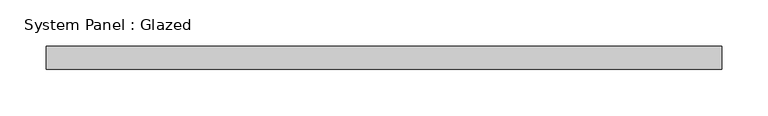
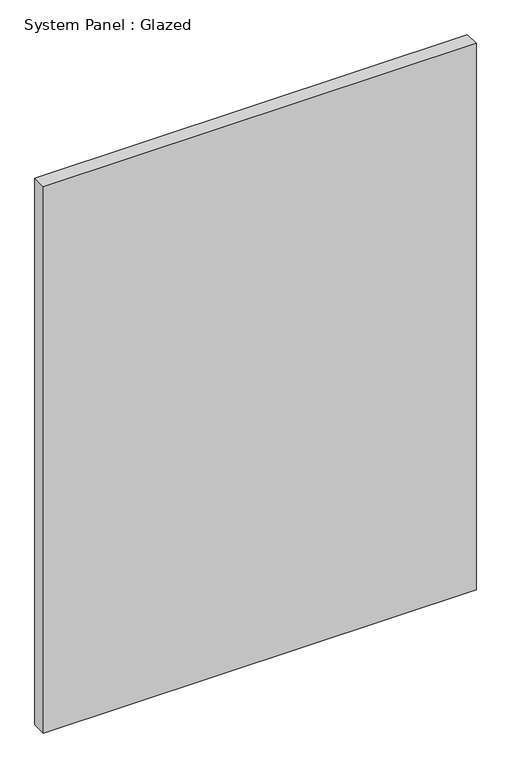
"""IFC4 building model written with IfcOpenShell, lengths in millimetres: plate geometry, System Panel : Glazed."""

from ifc_helpers import new_model, si_unit, origin, origin_with_axes, place, context, project, spatial, polyline, outline, extrude, source, transform, mapped, element, save


def system_panel_glazed_74337a84(model_context):
    return source(origin(), model_context, "Body", "SweptSolid", [
        extrude(outline(polyline([(365.0, 24.5), (-365.0, 24.5), (-365.0, 49.5), (365.0, 49.5), (365.0, 24.5)])), origin_with_axes(), (0.0, 0.0, 1.0), 975.0),
    ])


if __name__ == "__main__":
    model = new_model("IFC4")
    model_context = context("Model", 3, world=origin())
    ifc_project = project(units=[si_unit("LENGTHUNIT", "METRE", prefix="MILLI")], contexts=[model_context])
    site = spatial("IfcSite", under=ifc_project)
    building = spatial("IfcBuilding", under=site)
    placement = place(None, origin())
    system_panel_glazed_shape = system_panel_glazed_74337a84(model_context)
    element("IfcPlate", 1, ObjectType="System Panel : Glazed", at=placement, inside=building, context=model_context, shape_type="MappedRepresentation", body=[
        mapped(system_panel_glazed_shape, transform((0.0, 0.0, 0.0), x_axis=(1.0, 0.0, 0.0), y_axis=(0.0, 1.0, 0.0), z_axis=(0.0, 0.0, 1.0))),
    ])
    save(model, "model.ifc")

# Revit data of these elements
# Element 1 (IfcPlate, "System Panel : Glazed")
#   Materials on its faces: "Glass"
# Materials
#   "Glass": class "Glass", colour RGB 218 227 224, transparency 0.85, Description = "Soda Lime Glass", Cost = 0
